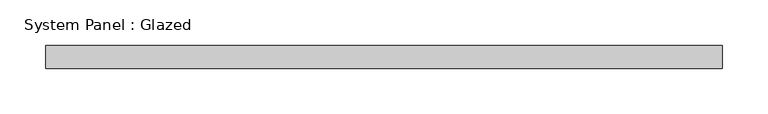
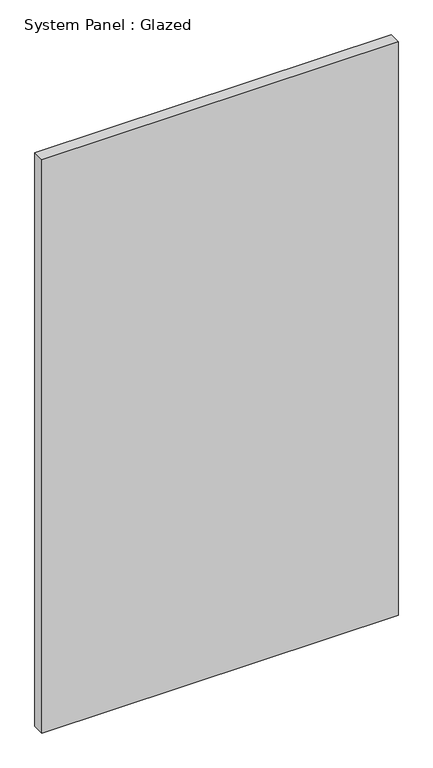
"""IFC4 building model written with IfcOpenShell, lengths in millimetres: plate geometry, System Panel : Glazed."""

from ifc_helpers import new_model, si_unit, origin, origin_with_axes, place, context, project, spatial, polyline, outline, extrude, source, transform, mapped, element, save


def system_panel_glazed_bebac94d(model_context):
    return source(origin(), model_context, "Body", "SweptSolid", [
        extrude(outline(polyline([(371.475, 19.05), (-371.475, 19.05), (-371.475, 44.45), (371.475, 44.45), (371.475, 19.05)])), origin_with_axes(), (0.0, 0.0, 1.0), 1264.4079139),
    ])


if __name__ == "__main__":
    model = new_model("IFC4")
    model_context = context("Model", 3, world=origin())
    ifc_project = project(units=[si_unit("LENGTHUNIT", "METRE", prefix="MILLI")], contexts=[model_context])
    site = spatial("IfcSite", under=ifc_project)
    building = spatial("IfcBuilding", under=site)
    placement = place(None, origin())
    system_panel_glazed_shape = system_panel_glazed_bebac94d(model_context)
    element("IfcPlate", 1, ObjectType="System Panel : Glazed", at=placement, inside=building, context=model_context, shape_type="MappedRepresentation", body=[
        mapped(system_panel_glazed_shape, transform((0.0, 0.0, 0.0), x_axis=(1.0, 0.0, 0.0), y_axis=(0.0, 1.0, 0.0), z_axis=(0.0, 0.0, 1.0))),
    ])
    save(model, "model.ifc")

# Revit data of these elements
# Type "System Panel : Glazed"
#   Construction Type Id = "GSP4R"
#   Analytic Construction = "1/8 in Pilkington single glazing"
#   Visual Light Transmittance = 0.9
#   Solar Heat Gain Coefficient = 0.86
#   Heat Transfer Coefficient (U) = 1.18115 BTU/(h·ft²·°F)
#   Define Thermal Properties by = 1
# Element 1 (IfcPlate, "System Panel : Glazed")
#   Materials on its faces: "Glass"
# Materials
#   "Glass": class "Glass", colour RGB 0 128 192, transparency 0.75, Description = "Soda Lime Glass", Cost = 0
